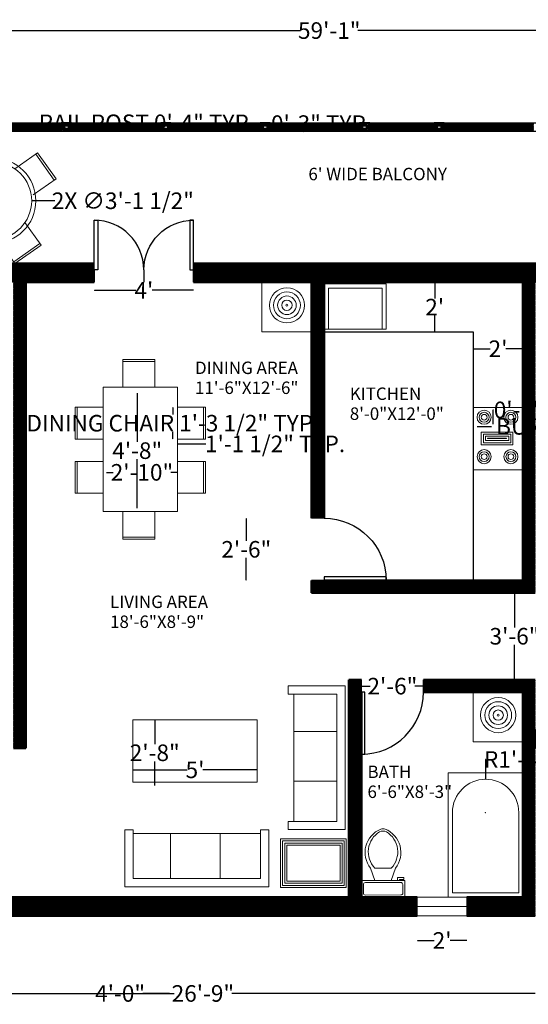
# Model space of a CAD drawing. Units: inches. Extents: x 348 to 1197, y 2602 to 3078.
# Tile 2 of 4: x 604 to 850, y 2602 to 3078. Entities that reach past the tile are written whole.
import ezdxf

# ---------------------------------------------------------------- set-up
doc = ezdxf.new("R2010")
doc.units = ezdxf.units.IN
doc.header["$MEASUREMENT"] = 0
for name, color, linetype, lineweight in [('A-ANNO-DIMS', 20, 'Continuous', 18), ('A-AREA-IDEN', 104, 'Continuous', 18), ('A-EQPM', 8, 'Continuous', 18), ('A-FLOR-CASE', 5, 'Continuous', 25), ('A-FLOR-FIXT', 9, 'Continuous', 18), ('A-WALL-PATT', 250, 'Continuous', 13), ('balcony', 201, 'Continuous', 25), ('doors', 1, 'Continuous', 25), ('sofa', 3, 'Continuous', 18), ('table', 6, 'Continuous', 18), ('walls', 4, 'Continuous', 50), ('windows', 2, 'Continuous', 18)]:
    doc.layers.add(name, color=color, linetype=linetype, lineweight=lineweight)
doc.styles.get("Standard").update_dxf_attribs({"font": 'arial.ttf'})
doc.dimstyles.get("Standard").update_dxf_attribs({"dimtxt": 8, "dimasz": 0.18, "dimexe": 0.18, "dimexo": 0.0625, "dimgap": 0.09, "dimtad": 0, "dimtih": 1, "dimtoh": 1, "dimdec": 0, "dimzin": 0, "dimdsep": 46, "dimlunit": 3, "dimtxsty": 'Standard', "dimblk": 'DOT', "dimcen": 0.09, "dimse1": 1, "dimse2": 1, "dimadec": 0, "dimazin": 0, "dimtfac": 1, "dimtdec": 0, "dimtofl": 0, "dimtmove": 0, "dimatfit": 3, "dimfxl": 1, "dimtolj": 1, "dimtzin": 0, "dimarcsym": 0})

# ---------------------------------------------------------------- blocks, each defined once
blk = doc.blocks.new('*U10')
for p, q in [((0, 0), (0, -6)), ((30, 0), (30, -6))]:
    blk.add_line(p, q)
blk.add_lwpolyline([(0, 0), (0, 30), (1.75, 30), (1.75, 0)], close=True)
blk.add_arc((0, 0), 30, 0, 90)
blk = doc.blocks.new('*U6')
for p, q in [((0, 0), (0, 6)), ((30, 0), (30, 6))]:
    blk.add_line(p, q)
blk.add_lwpolyline([(0, 0), (0, -30), (1.75, -30), (1.75, 0)], close=True)
blk.add_arc((0, 0), 30, 270, 0)
blk = doc.blocks.new('*U12')
for p, q in [((-4.02, 7.99), (-6.03, 13.99)), ((-4.03, 13.99), (3.97, 14.01)), ((3.98, 8.01), (5.97, 14.01)), ((6.98, 9.51), (9.98, 9.52)), ((6.98, 8.01), (6.98, 9.51)), ((9.98, 9.52), (9.98, 8.52)), ((-9.51, 5.98), (-9.5, 1.98)), ((9.98, 8.52), (7.98, 8.52)), ((7.98, 8.52), (7.98, 8.02))]:
    blk.add_line(p, q)
blk.add_lwpolyline([(-10.51, 7.98), (-10.5, -0.02), (10.5, 0.02), (10.48, 8.02)], close=True)
for points in [[(8.49, 7.02), (-8.51, 6.98)], [(9.5, 2.02), (9.49, 6.02)], [(-8.5, 0.98), (8.5, 1.02)]]:
    blk.add_lwpolyline(points)
for centre, radius, start, end in [((3.48, 21.59), 12.17, 112.136, 218.6382), ((4.16, 21.83), 11.33, 121.1605, 223.7396), ((-0.05, 27.88), 4, 65.8394, 114.3757), ((-0.05, 29), 4, 74.9681, 105.247), ((-3.56, 21.57), 12.17, 321.5766, 68.079), ((-4.24, 21.81), 11.33, 316.4753, 59.0544), ((-8.64, 6.11), 0.884, 81.9774, 188.2376), ((8.61, 6.14), 0.884, 351.9774, 98.2376), ((-8.63, 1.86), 0.884, 171.9774, 278.2376), ((8.62, 1.89), 0.884, 261.9774, 8.2376)]:
    blk.add_arc(centre, radius, start, end)
blk = doc.blocks.new('*U14')
at = {"layer": 'table'}
for p, q in [((-7.7, -6.73), (-7.7, 6.73)), ((-7.7, 6.73), (7.7, 6.73)), ((-7.7, 5.73), (7.7, 5.73)), ((7.7, 6.73), (7.7, -6.73))]:
    blk.add_line(p, q, dxfattribs=at)
blk = doc.blocks.new('*U15')
at = {"layer": 'table', "transparency": 16777216}
blk.add_blockref('*U14', (596.31, 3015.18), dxfattribs=at)
for p, rotation in [((570.95, 2992.17), 90), ((619.32, 2989.82), 270), ((593.96, 2966.81), 180)]:
    blk.add_blockref('*U14', p, dxfattribs=dict(at, rotation=rotation))
blk = doc.blocks.new('*U18')
for p, q in [((0, 0), (0, -6)), ((24, 0), (24, -6))]:
    blk.add_line(p, q)
blk.add_lwpolyline([(0, 0), (0, 24), (1.75, 24), (1.75, 0)], close=True)
blk.add_arc((0, 0), 24, 0, 90)
blk = doc.blocks.new('_Dot')
at = {"color": 0, "linetype": 'ByBlock', "lineweight": -2}
blk.add_line((-0.5, 0), (-1, 0), dxfattribs=at)
at = {"color": 0, "linetype": 'ByBlock', "const_width": 0.5}
blk.add_lwpolyline([(-0.25, 0, 1), (0.25, 0, 1)], format="xyb", close=True, dxfattribs=at)
blk = doc.blocks.new('*D25')
at = {"layer": 'A-ANNO-DIMS', "color": 0, "lineweight": -2, "transparency": 16777216}
for p, q in [((769.5, 2756.1), (773.53, 2756.1)), ((799.14, 2756.1), (795.11, 2756.1))]:
    blk.add_line(p, q, dxfattribs=at)
at = {"layer": 'Defpoints', "color": 0, "transparency": 16777216}
for p in [(769.32, 2756.1), (769.32, 2756.1), (799.32, 2756.2)]:
    blk.add_point(p, dxfattribs=at)
at = {"layer": 'A-ANNO-DIMS', "color": 0, "lineweight": -2, "transparency": 16777216, "xscale": 0.18, "yscale": 0.18, "zscale": 0.18, "rotation": 180}
blk.add_blockref('_Dot', (769.32, 2756.1), dxfattribs=at)
at = {"layer": 'A-ANNO-DIMS', "color": 0, "lineweight": -2, "transparency": 16777216, "xscale": 0.18, "yscale": 0.18, "zscale": 0.18}
blk.add_blockref('_Dot', (799.32, 2756.1), dxfattribs=at)
at = {"layer": 'A-ANNO-DIMS', "color": 0, "transparency": 16777216, "insert": (784.32, 2756.1), "char_height": 8, "attachment_point": 5}
blk.add_mtext('\\A1;2\'-6"', dxfattribs=at)
blk = doc.blocks.new('*D26')
at = {"layer": 'A-ANNO-DIMS', "color": 0, "lineweight": -2, "transparency": 16777216}
for p, q in [((843.28, 2801.02), (843.28, 2784.38)), ((843.28, 2759.38), (843.28, 2776.03))]:
    blk.add_line(p, q, dxfattribs=at)
at = {"layer": 'Defpoints', "color": 0, "transparency": 16777216}
for p in [(843.28, 2801.2), (843.28, 2759.2), (843.28, 2759.2)]:
    blk.add_point(p, dxfattribs=at)
at = {"layer": 'A-ANNO-DIMS', "color": 0, "lineweight": -2, "transparency": 16777216, "xscale": 0.18, "yscale": 0.18, "zscale": 0.18}
for p, rotation in [((843.28, 2801.2), 90), ((843.28, 2759.2), 270)]:
    blk.add_blockref('_Dot', p, dxfattribs=dict(at, rotation=rotation))
at = {"layer": 'A-ANNO-DIMS', "color": 0, "transparency": 16777216, "insert": (843.28, 2780.2), "char_height": 8, "attachment_point": 5}
blk.add_mtext('\\A1;3\'-6"', dxfattribs=at)
blk = doc.blocks.new('*D30')
at = {"layer": 'A-ANNO-DIMS', "color": 0, "lineweight": -2, "transparency": 16777216}
for p, q in [((640.5, 2947.32), (660.39, 2947.32)), ((688.14, 2947.32), (668.25, 2947.32))]:
    blk.add_line(p, q, dxfattribs=at)
at = {"layer": 'Defpoints', "color": 0, "transparency": 16777216}
for p in [(640.32, 2951.2), (688.32, 2951.2), (688.32, 2947.32)]:
    blk.add_point(p, dxfattribs=at)
at = {"layer": 'A-ANNO-DIMS', "color": 0, "lineweight": -2, "transparency": 16777216, "xscale": 0.18, "yscale": 0.18, "zscale": 0.18, "rotation": 180}
blk.add_blockref('_Dot', (640.32, 2947.32), dxfattribs=at)
at = {"layer": 'A-ANNO-DIMS', "color": 0, "lineweight": -2, "transparency": 16777216, "xscale": 0.18, "yscale": 0.18, "zscale": 0.18}
blk.add_blockref('_Dot', (688.32, 2947.32), dxfattribs=at)
at = {"layer": 'A-ANNO-DIMS', "color": 0, "transparency": 16777216, "insert": (664.32, 2947.32), "char_height": 8, "attachment_point": 5}
blk.add_mtext("\\A1;4'", dxfattribs=at)
blk = doc.blocks.new('*D31')
at = {"layer": 'A-ANNO-DIMS', "color": 0, "lineweight": -2, "transparency": 16777216}
for p, q in [((804.74, 2951.02), (804.74, 2943.31)), ((804.74, 2927.38), (804.74, 2935.1))]:
    blk.add_line(p, q, dxfattribs=at)
at = {"layer": 'Defpoints', "color": 0, "transparency": 16777216}
for p in [(798.02, 2951.2), (804.74, 2951.2), (798.02, 2927.2)]:
    blk.add_point(p, dxfattribs=at)
at = {"layer": 'A-ANNO-DIMS', "color": 0, "lineweight": -2, "transparency": 16777216, "xscale": 0.18, "yscale": 0.18, "zscale": 0.18}
for p, rotation in [((804.74, 2951.2), 90), ((804.74, 2927.2), 270)]:
    blk.add_blockref('_Dot', p, dxfattribs=dict(at, rotation=rotation))
at = {"layer": 'A-ANNO-DIMS', "color": 0, "transparency": 16777216, "insert": (804.74, 2939.2), "char_height": 8, "attachment_point": 5}
blk.add_mtext("\\A1;2'", dxfattribs=at)
blk = doc.blocks.new('*D32')
at = {"layer": 'A-ANNO-DIMS', "color": 0, "lineweight": -2, "transparency": 16777216}
for p, q in [((823.5, 2919.1), (831.48, 2919.1)), ((847.14, 2919.1), (839.16, 2919.1))]:
    blk.add_line(p, q, dxfattribs=at)
at = {"layer": 'Defpoints', "color": 0, "transparency": 16777216}
for p in [(823.32, 2927.2), (847.32, 2927.2), (847.32, 2919.1)]:
    blk.add_point(p, dxfattribs=at)
at = {"layer": 'A-ANNO-DIMS', "color": 0, "lineweight": -2, "transparency": 16777216, "xscale": 0.18, "yscale": 0.18, "zscale": 0.18, "rotation": 180}
blk.add_blockref('_Dot', (823.32, 2919.1), dxfattribs=at)
at = {"layer": 'A-ANNO-DIMS', "color": 0, "lineweight": -2, "transparency": 16777216, "xscale": 0.18, "yscale": 0.18, "zscale": 0.18}
blk.add_blockref('_Dot', (847.32, 2919.1), dxfattribs=at)
at = {"layer": 'A-ANNO-DIMS', "color": 0, "transparency": 16777216, "insert": (835.32, 2919.1), "char_height": 8, "attachment_point": 5}
blk.add_mtext("\\A1;2'", dxfattribs=at)
blk = doc.blocks.new('*D35')
at = {"layer": 'A-ANNO-DIMS', "color": 0, "lineweight": -2, "transparency": 16777216}
for p, q in [((659.18, 2715.69), (685.23, 2715.69)), ((718.82, 2715.69), (692.77, 2715.69))]:
    blk.add_line(p, q, dxfattribs=at)
at = {"layer": 'Defpoints', "color": 0, "transparency": 16777216}
for p in [(659, 2715.69), (659, 2709.77), (719, 2709.77)]:
    blk.add_point(p, dxfattribs=at)
at = {"layer": 'A-ANNO-DIMS', "color": 0, "lineweight": -2, "transparency": 16777216, "xscale": 0.18, "yscale": 0.18, "zscale": 0.18, "rotation": 180}
blk.add_blockref('_Dot', (659, 2715.69), dxfattribs=at)
at = {"layer": 'A-ANNO-DIMS', "color": 0, "lineweight": -2, "transparency": 16777216, "xscale": 0.18, "yscale": 0.18, "zscale": 0.18}
blk.add_blockref('_Dot', (719, 2715.69), dxfattribs=at)
at = {"layer": 'A-ANNO-DIMS', "color": 0, "transparency": 16777216, "insert": (689, 2715.69), "char_height": 8, "attachment_point": 5}
blk.add_mtext("\\A1;5'", dxfattribs=at)
blk = doc.blocks.new('*D36')
at = {"layer": 'A-ANNO-DIMS', "color": 0, "lineweight": -2, "transparency": 16777216}
for p, q in [((669.57, 2739.59), (669.57, 2728.1)), ((669.57, 2708.25), (669.57, 2719.75))]:
    blk.add_line(p, q, dxfattribs=at)
at = {"layer": 'Defpoints', "color": 0, "transparency": 16777216}
for p in [(669.57, 2739.77), (675.29, 2739.77), (673.39, 2708.07)]:
    blk.add_point(p, dxfattribs=at)
at = {"layer": 'A-ANNO-DIMS', "color": 0, "lineweight": -2, "transparency": 16777216, "xscale": 0.18, "yscale": 0.18, "zscale": 0.18}
for p, rotation in [((669.57, 2739.77), 90), ((669.57, 2708.07), 270)]:
    blk.add_blockref('_Dot', p, dxfattribs=dict(at, rotation=rotation))
at = {"layer": 'A-ANNO-DIMS', "color": 0, "transparency": 16777216, "insert": (669.57, 2723.92), "char_height": 8, "attachment_point": 5}
blk.add_mtext('\\A1;2\'-8"', dxfattribs=at)
blk = doc.blocks.new('*D37')
at = {"layer": 'A-ANNO-DIMS', "color": 0, "lineweight": -2, "transparency": 16777216}
for p, q in [((646.36, 2859.39), (649.5, 2859.39)), ((680.44, 2859.39), (677.3, 2859.39))]:
    blk.add_line(p, q, dxfattribs=at)
at = {"layer": 'Defpoints', "color": 0, "transparency": 16777216}
for p in [(646.18, 2869.07), (680.62, 2869.07), (646.18, 2859.39)]:
    blk.add_point(p, dxfattribs=at)
at = {"layer": 'A-ANNO-DIMS', "color": 0, "lineweight": -2, "transparency": 16777216, "xscale": 0.18, "yscale": 0.18, "zscale": 0.18, "rotation": 180}
blk.add_blockref('_Dot', (646.18, 2859.39), dxfattribs=at)
at = {"layer": 'A-ANNO-DIMS', "color": 0, "lineweight": -2, "transparency": 16777216, "xscale": 0.18, "yscale": 0.18, "zscale": 0.18}
blk.add_blockref('_Dot', (680.62, 2859.39), dxfattribs=at)
at = {"layer": 'A-ANNO-DIMS', "color": 0, "transparency": 16777216, "insert": (663.4, 2859.39), "char_height": 8, "attachment_point": 5}
blk.add_mtext('\\A1;2\'-10"', dxfattribs=at)
blk = doc.blocks.new('*D38')
at = {"layer": 'A-ANNO-DIMS', "color": 0, "lineweight": -2, "transparency": 16777216}
for p, q in [((661.12, 2897.52), (661.12, 2874.05)), ((661.12, 2842.23), (661.12, 2865.7))]:
    blk.add_line(p, q, dxfattribs=at)
at = {"layer": 'Defpoints', "color": 0, "transparency": 16777216}
for p in [(657.08, 2897.7), (661.12, 2897.7), (657.08, 2842.05)]:
    blk.add_point(p, dxfattribs=at)
at = {"layer": 'A-ANNO-DIMS', "color": 0, "lineweight": -2, "transparency": 16777216, "xscale": 0.18, "yscale": 0.18, "zscale": 0.18}
for p, rotation in [((661.12, 2897.7), 90), ((661.12, 2842.05), 270)]:
    blk.add_blockref('_Dot', p, dxfattribs=dict(at, rotation=rotation))
at = {"layer": 'A-ANNO-DIMS', "color": 0, "transparency": 16777216, "insert": (661.12, 2869.87), "char_height": 8, "attachment_point": 5}
blk.add_mtext('\\A1;4\'-8"', dxfattribs=at)
blk = doc.blocks.new('*D39')
at = {"layer": 'A-ANNO-DIMS', "color": 0, "lineweight": -2, "transparency": 16777216}
for p, q in [((796.5, 2633.23), (804.48, 2633.23)), ((820.14, 2633.23), (812.16, 2633.23))]:
    blk.add_line(p, q, dxfattribs=at)
at = {"layer": 'Defpoints', "color": 0, "transparency": 16777216}
for p in [(796.32, 2645.2), (820.32, 2645.2), (820.32, 2633.23)]:
    blk.add_point(p, dxfattribs=at)
at = {"layer": 'A-ANNO-DIMS', "color": 0, "lineweight": -2, "transparency": 16777216, "xscale": 0.18, "yscale": 0.18, "zscale": 0.18, "rotation": 180}
blk.add_blockref('_Dot', (796.32, 2633.23), dxfattribs=at)
at = {"layer": 'A-ANNO-DIMS', "color": 0, "lineweight": -2, "transparency": 16777216, "xscale": 0.18, "yscale": 0.18, "zscale": 0.18}
blk.add_blockref('_Dot', (820.32, 2633.23), dxfattribs=at)
at = {"layer": 'A-ANNO-DIMS', "color": 0, "transparency": 16777216, "insert": (808.32, 2633.23), "char_height": 8, "attachment_point": 5}
blk.add_mtext("\\A1;2'", dxfattribs=at)
blk = doc.blocks.new('RAIL-POST-CORE')
for points in [[(0, 0), (3, 0), (3, 3.9), (0, 3.9)], [(0.5, 0.5), (2.5, 0.5), (2.5, 3.4), (0.5, 3.4)], [(1, 1), (2, 1), (2, 2.9), (1, 2.9)]]:
    blk.add_lwpolyline(points, close=True)
blk = doc.blocks.new('DINING-CHAIR')
for p, q in [((0, 0), (0, 13.45)), ((0, 13.45), (15.39, 13.45)), ((0, 12.45), (15.39, 12.45)), ((15.39, 13.45), (15.39, 0))]:
    blk.add_line(p, q)
blk = doc.blocks.new('BALCONY-TABLE-ROUND')
for radius in [20.64, 18.64]:
    blk.add_circle((20.64, 20.64), radius)
blk = doc.blocks.new('BASIN-ROUND')
for radius in [8.49, 8.49, 8.49, 6.49, 4.49, 4.49, 2.49, 0.487]:
    blk.add_circle((8.49, 8.49), radius)
blk = doc.blocks.new('COOKTOP-BURNER')
for radius in [3.39, 2.39, 1.39]:
    blk.add_circle((3.39, 3.39), radius)
blk = doc.blocks.new('*D50')
at = {"layer": 'A-ANNO-DIMS', "color": 0, "lineweight": -2, "transparency": 16777216}
for p, q in [((720.96, 3028.25), (720.78, 3028.25)), ((724.68, 3028.25), (721.14, 3028.25))]:
    blk.add_line(p, q, dxfattribs=at)
at = {"layer": 'Defpoints', "color": 0, "transparency": 16777216}
for p in [(720.96, 3028.25), (720.96, 3027.67), (724.86, 3027.67)]:
    blk.add_point(p, dxfattribs=at)
at = {"layer": 'A-ANNO-DIMS', "color": 0, "lineweight": -2, "transparency": 16777216, "xscale": 0.18, "yscale": 0.18, "zscale": 0.18}
for p, rotation in [((720.96, 3028.25), 180.0000000000133), ((724.86, 3028.25), 1.33493e-11)]:
    blk.add_blockref('_Dot', p, dxfattribs=dict(at, rotation=rotation))
at = {"layer": 'A-ANNO-DIMS', "color": 0, "transparency": 16777216, "insert": (665.78, 3028.25), "char_height": 8, "attachment_point": 5}
blk.add_mtext('\\A1;RAIL POST 0\'-4" TYP.', dxfattribs=at)
blk = doc.blocks.new('*D51')
at = {"layer": 'A-ANNO-DIMS', "color": 0, "lineweight": -2, "transparency": 16777216}
for p, q in [((725.45, 3027.67), (725.45, 3027.85)), ((725.45, 3027.85), (725.63, 3027.85)), ((725.45, 3024.85), (725.45, 3027.49))]:
    blk.add_line(p, q, dxfattribs=at)
at = {"layer": 'Defpoints', "color": 0, "transparency": 16777216}
for p in [(724.86, 3027.67), (725.45, 3027.67), (724.86, 3024.67)]:
    blk.add_point(p, dxfattribs=at)
at = {"layer": 'A-ANNO-DIMS', "color": 0, "lineweight": -2, "transparency": 16777216, "xscale": 0.18, "yscale": 0.18, "zscale": 0.18}
for p, rotation in [((725.45, 3027.67), 90), ((725.45, 3024.67), 270)]:
    blk.add_blockref('_Dot', p, dxfattribs=dict(at, rotation=rotation))
at = {"layer": 'A-ANNO-DIMS', "color": 0, "transparency": 16777216, "insert": (750.1, 3027.85), "char_height": 8, "attachment_point": 5}
blk.add_mtext('\\A1;0\'-3" TYP.', dxfattribs=at)
blk = doc.blocks.new('*D56')
at = {"layer": 'A-ANNO-DIMS', "color": 0, "lineweight": -2, "transparency": 16777216}
for p, q in [((678.31, 2890.64), (678.31, 2887.35)), ((678.31, 2875.61), (678.31, 2878.89))]:
    blk.add_line(p, q, dxfattribs=at)
at = {"layer": 'Defpoints', "color": 0, "transparency": 16777216}
for p in [(680.62, 2890.82), (678.31, 2875.43), (680.62, 2875.43)]:
    blk.add_point(p, dxfattribs=at)
at = {"layer": 'A-ANNO-DIMS', "color": 0, "lineweight": -2, "transparency": 16777216, "xscale": 0.18, "yscale": 0.18, "zscale": 0.18}
for p, rotation in [((678.31, 2890.82), 90), ((678.31, 2875.43), 270)]:
    blk.add_blockref('_Dot', p, dxfattribs=dict(at, rotation=rotation))
at = {"layer": 'A-ANNO-DIMS', "color": 0, "transparency": 16777216, "insert": (678.31, 2883.12), "char_height": 8, "attachment_point": 5}
blk.add_mtext('\\A1;DINING CHAIR 1\'-3 1/2" TYP.', dxfattribs=at)
blk = doc.blocks.new('*D57')
at = {"layer": 'A-ANNO-DIMS', "color": 0, "lineweight": -2, "transparency": 16777216}
for p, q in [((680.8, 2873.12), (693.89, 2873.12)), ((694.07, 2873.12), (694.25, 2873.12))]:
    blk.add_line(p, q, dxfattribs=at)
at = {"layer": 'Defpoints', "color": 0, "transparency": 16777216}
for p in [(680.62, 2875.43), (694.07, 2875.43), (694.07, 2873.12)]:
    blk.add_point(p, dxfattribs=at)
at = {"layer": 'A-ANNO-DIMS', "color": 0, "lineweight": -2, "transparency": 16777216, "xscale": 0.18, "yscale": 0.18, "zscale": 0.18, "rotation": 180}
blk.add_blockref('_Dot', (680.62, 2873.12), dxfattribs=at)
at = {"layer": 'A-ANNO-DIMS', "color": 0, "lineweight": -2, "transparency": 16777216, "xscale": 0.18, "yscale": 0.18, "zscale": 0.18}
blk.add_blockref('_Dot', (694.07, 2873.12), dxfattribs=at)
at = {"layer": 'A-ANNO-DIMS', "color": 0, "transparency": 16777216, "insert": (727.67, 2873.12), "char_height": 8, "attachment_point": 5}
blk.add_mtext('\\A1;1\'-1 1/2" TYP.', dxfattribs=at)
blk = doc.blocks.new('*D62')
at = {"layer": 'A-ANNO-DIMS', "color": 0, "lineweight": -2, "transparency": 16777216}
for p, q in [((825.4, 2881.58), (831.83, 2881.58)), ((832.01, 2881.58), (832.19, 2881.58))]:
    blk.add_line(p, q, dxfattribs=at)
at = {"layer": 'Defpoints', "color": 0, "transparency": 16777216}
for p in [(825.22, 2882.6), (832.01, 2882.6), (832.01, 2881.58)]:
    blk.add_point(p, dxfattribs=at)
at = {"layer": 'A-ANNO-DIMS', "color": 0, "lineweight": -2, "transparency": 16777216, "xscale": 0.18, "yscale": 0.18, "zscale": 0.18, "rotation": 180}
blk.add_blockref('_Dot', (825.22, 2881.58), dxfattribs=at)
at = {"layer": 'A-ANNO-DIMS', "color": 0, "lineweight": -2, "transparency": 16777216, "xscale": 0.18, "yscale": 0.18, "zscale": 0.18}
blk.add_blockref('_Dot', (832.01, 2881.58), dxfattribs=at)
at = {"layer": 'A-ANNO-DIMS', "color": 0, "transparency": 16777216, "insert": (881.63, 2881.58), "char_height": 8, "attachment_point": 5}
blk.add_mtext('\\A1;BURNER 0\'-7" TYP.', dxfattribs=at)
blk = doc.blocks.new('*D63')
at = {"layer": 'A-ANNO-DIMS', "color": 0, "lineweight": -2, "transparency": 16777216}
for p, q in [((833.03, 2889.38), (833.03, 2889.56)), ((833.03, 2889.56), (833.21, 2889.56)), ((833.03, 2882.78), (833.03, 2889.2))]:
    blk.add_line(p, q, dxfattribs=at)
at = {"layer": 'Defpoints', "color": 0, "transparency": 16777216}
for p in [(832.01, 2889.38), (833.03, 2889.38), (832.01, 2882.6)]:
    blk.add_point(p, dxfattribs=at)
at = {"layer": 'A-ANNO-DIMS', "color": 0, "lineweight": -2, "transparency": 16777216, "xscale": 0.18, "yscale": 0.18, "zscale": 0.18}
for p, rotation in [((833.03, 2889.38), 90), ((833.03, 2882.6), 270)]:
    blk.add_blockref('_Dot', p, dxfattribs=dict(at, rotation=rotation))
at = {"layer": 'A-ANNO-DIMS', "color": 0, "transparency": 16777216, "insert": (857.68, 2889.56), "char_height": 8, "attachment_point": 5}
blk.add_mtext('\\A1;0\'-7" TYP.', dxfattribs=at)
blk = doc.blocks.new('*D68')
at = {"layer": 'A-ANNO-DIMS', "color": 0, "lineweight": -2, "transparency": 16777216}
for p, q in [((399.5, 3072.8), (739.99, 3072.8)), ((1108.14, 3072.8), (767.65, 3072.8))]:
    blk.add_line(p, q, dxfattribs=at)
at = {"layer": 'Defpoints', "color": 0, "transparency": 16777216}
for p in [(1108.32, 3072.8), (1108.32, 3028.2), (399.32, 3018.2)]:
    blk.add_point(p, dxfattribs=at)
at = {"layer": 'A-ANNO-DIMS', "color": 0, "lineweight": -2, "transparency": 16777216, "xscale": 0.18, "yscale": 0.18, "zscale": 0.18, "rotation": 180}
blk.add_blockref('_Dot', (399.32, 3072.8), dxfattribs=at)
at = {"layer": 'A-ANNO-DIMS', "color": 0, "lineweight": -2, "transparency": 16777216, "xscale": 0.18, "yscale": 0.18, "zscale": 0.18}
blk.add_blockref('_Dot', (1108.32, 3072.8), dxfattribs=at)
at = {"layer": 'A-ANNO-DIMS', "color": 0, "transparency": 16777216, "insert": (753.82, 3072.8), "char_height": 8, "attachment_point": 5}
blk.add_mtext('\\A1;59\'-1"', dxfattribs=at)
blk = doc.blocks.new('*D72')
at = {"layer": 'A-ANNO-DIMS', "color": 0, "lineweight": -2, "transparency": 16777216}
for p, q in [((532.5, 2607.65), (678.92, 2607.65)), ((853.14, 2607.65), (706.72, 2607.65))]:
    blk.add_line(p, q, dxfattribs=at)
at = {"layer": 'Defpoints', "color": 0, "transparency": 16777216}
for p in [(532.32, 2645.2), (853.32, 2645.2), (853.32, 2607.65)]:
    blk.add_point(p, dxfattribs=at)
at = {"layer": 'A-ANNO-DIMS', "color": 0, "lineweight": -2, "transparency": 16777216, "xscale": 0.18, "yscale": 0.18, "zscale": 0.18, "rotation": 180}
blk.add_blockref('_Dot', (532.32, 2607.65), dxfattribs=at)
at = {"layer": 'A-ANNO-DIMS', "color": 0, "lineweight": -2, "transparency": 16777216, "xscale": 0.18, "yscale": 0.18, "zscale": 0.18}
blk.add_blockref('_Dot', (853.32, 2607.65), dxfattribs=at)
at = {"layer": 'A-ANNO-DIMS', "color": 0, "transparency": 16777216, "insert": (692.82, 2607.65), "char_height": 8, "attachment_point": 5}
blk.add_mtext('\\A1;26\'-9"', dxfattribs=at)
blk = doc.blocks.new('*D76')
at = {"layer": 'A-ANNO-DIMS', "color": 0, "lineweight": -2, "transparency": 16777216}
for p, q in [((629.04, 2607.65), (641.98, 2607.65)), ((676.68, 2607.65), (663.75, 2607.65))]:
    blk.add_line(p, q, dxfattribs=at)
at = {"layer": 'Defpoints', "color": 0, "transparency": 16777216}
for p in [(628.86, 3024.67), (676.86, 3024.67), (676.86, 2607.65)]:
    blk.add_point(p, dxfattribs=at)
at = {"layer": 'A-ANNO-DIMS', "color": 0, "lineweight": -2, "transparency": 16777216, "xscale": 0.18, "yscale": 0.18, "zscale": 0.18, "rotation": 180}
blk.add_blockref('_Dot', (628.86, 2607.65), dxfattribs=at)
at = {"layer": 'A-ANNO-DIMS', "color": 0, "lineweight": -2, "transparency": 16777216, "xscale": 0.18, "yscale": 0.18, "zscale": 0.18}
blk.add_blockref('_Dot', (676.86, 2607.65), dxfattribs=at)
at = {"layer": 'A-ANNO-DIMS', "color": 0, "transparency": 16777216, "insert": (652.86, 2607.65), "char_height": 8, "attachment_point": 5}
blk.add_mtext('\\A1;4\'-0"', dxfattribs=at)
blk = doc.blocks.new('*D77')
at = {"layer": 'A-ANNO-DIMS', "color": 0, "lineweight": -2, "transparency": 16777216}
for p, q in [((713.77, 2837.02), (713.77, 2826.38)), ((713.77, 2807.38), (713.77, 2818.03))]:
    blk.add_line(p, q, dxfattribs=at)
at = {"layer": 'Defpoints', "color": 0, "transparency": 16777216}
for p in [(713.77, 2837.2), (751.32, 2837.2), (751.32, 2807.2)]:
    blk.add_point(p, dxfattribs=at)
at = {"layer": 'A-ANNO-DIMS', "color": 0, "lineweight": -2, "transparency": 16777216, "xscale": 0.18, "yscale": 0.18, "zscale": 0.18}
for p, rotation in [((713.77, 2837.2), 90), ((713.77, 2807.2), 270)]:
    blk.add_blockref('_Dot', p, dxfattribs=dict(at, rotation=rotation))
at = {"layer": 'A-ANNO-DIMS', "color": 0, "transparency": 16777216, "insert": (713.77, 2822.2), "char_height": 8, "attachment_point": 5}
blk.add_mtext('\\A1;2\'-6"', dxfattribs=at)
blk = doc.blocks.new('*D82')
at = {"layer": 'A-ANNO-DIMS', "color": 0, "lineweight": -2, "transparency": 16777216}
for p, q in [((591.41, 2990.59), (591.59, 2990.59)), ((591.5, 2990.5), (591.5, 2990.68)), ((621.33, 2990.59), (610.32, 2990.59))]:
    blk.add_line(p, q, dxfattribs=at)
at = {"layer": 'Defpoints', "color": 0, "transparency": 16777216}
for p in [(572.87, 2990.6), (610.14, 2990.59)]:
    blk.add_point(p, dxfattribs=at)
at = {"layer": 'A-ANNO-DIMS', "color": 0, "lineweight": -2, "transparency": 16777216, "xscale": 0.18, "yscale": 0.18, "zscale": 0.18, "rotation": 179.9894899347775}
blk.add_blockref('_Dot', (610.14, 2990.59), dxfattribs=at)
at = {"layer": 'A-ANNO-DIMS', "color": 0, "transparency": 16777216, "insert": (654.17, 2990.59), "char_height": 8, "attachment_point": 5}
blk.add_mtext('\\A1;2X ∅3\'-1 1/2"', dxfattribs=at)
blk = doc.blocks.new('*D83')
at = {"layer": 'A-ANNO-DIMS', "color": 0, "lineweight": -2, "transparency": 16777216}
for p, q in [((829.5, 2720.69), (829.32, 2720.69)), ((829.32, 2720.69), (829.32, 2711.27)), ((829.23, 2695.09), (829.41, 2695.09)), ((829.32, 2695), (829.32, 2695.18))]:
    blk.add_line(p, q, dxfattribs=at)
at = {"layer": 'Defpoints', "color": 0, "transparency": 16777216}
for p in [(829.32, 2711.09), (829.32, 2695.09)]:
    blk.add_point(p, dxfattribs=at)
at = {"layer": 'A-ANNO-DIMS', "color": 0, "lineweight": -2, "transparency": 16777216, "xscale": 0.18, "yscale": 0.18, "zscale": 0.18, "rotation": 269.9894074428831}
blk.add_blockref('_Dot', (829.32, 2711.09), dxfattribs=at)
at = {"layer": 'A-ANNO-DIMS', "color": 0, "transparency": 16777216, "insert": (844.05, 2720.69), "char_height": 8, "attachment_point": 5}
blk.add_mtext('\\A1;R1\'-4"', dxfattribs=at)

msp = doc.modelspace()

# ---------------------------------------------------------------- hatches: boundary and pattern name
at = {"layer": 'A-WALL-PATT'}
h = msp.add_hatch(dxfattribs=at)
h.set_pattern_fill('ANSI31', color=256, scale=1.5)
h.paths.add_polyline_path([(481.32, 2951.2), (509.32, 2951.2), (509.32, 2960.2), (505.32, 2960.2), (481.32, 2960.2), (481.32, 3018.2), (452.32, 3018.2), (452.32, 3009.2), (472.32, 3009.2), (472.32, 2943.2), (481.32, 2943.2)], flags=17)
h.paths.add_polyline_path([(428.32, 3018.2), (399.32, 3018.2), (399.32, 2904.2), (472.32, 2904.2), (472.32, 2726.2), (532.32, 2726.2), (532.32, 2696.2), (541.32, 2696.2), (541.32, 2726.2), (565.32, 2726.2), (565.32, 2735.2), (481.32, 2735.2), (481.32, 2758.72), (481.32, 2809.83), (481.31, 2809.83), (481.31, 2824.34), (481.31, 2884.34), (481.31, 2884.34), (481.31, 2898.86), (481.32, 2913.2), (472.32, 2913.2), (408.32, 2913.2), (408.32, 3009.2), (428.32, 3009.2)])
h.paths.add_polyline_path([(796.32, 2654.2), (769.32, 2654.2), (769.32, 2753.2), (769.32, 2759.2), (763.32, 2759.2), (763.32, 2735.2), (763.32, 2654.2), (541.32, 2654.2), (532.32, 2654.2), (532.32, 2645.2), (796.32, 2645.2)])
h.paths.add_polyline_path([(853.32, 2726.2), (1018.32, 2726.2), (1018.32, 2703.7), (1027.32, 2703.7), (1027.32, 2729.2), (1057.32, 2729.2), (1057.32, 2735.2), (919.32, 2735.2), (919.32, 2758.72), (919.32, 2765.2), (913.32, 2765.2), (913.32, 2735.2), (853.32, 2735.2), (853.32, 2759.2), (799.32, 2759.2), (799.32, 2753.2), (847.32, 2753.2), (847.32, 2654.2), (820.32, 2654.2), (820.32, 2645.2), (853.32, 2645.2)])
h.paths.add_polyline_path([(640.32, 2960.2), (577.32, 2960.2), (577.32, 2951.2), (601.32, 2951.2), (601.32, 2735.2), (601.32, 2726.2), (607.32, 2726.2), (607.32, 2951.2), (640.32, 2951.2)])
h.paths.add_polyline_path([(877.32, 2960.2), (688.32, 2960.2), (688.32, 2951.2), (745.32, 2951.2), (745.32, 2837.2), (751.32, 2837.2), (751.32, 2951.2), (847.32, 2951.2), (847.32, 2807.2), (751.32, 2807.2), (745.32, 2807.2), (745.32, 2801.2), (853.32, 2801.2), (853.32, 2807.2), (853.32, 2951.2), (877.32, 2951.2)])
h.paths.add_polyline_path([(1003.32, 2960.2), (949.32, 2960.2), (949.32, 2951.2), (973.32, 2951.2), (973.32, 2807.2), (906.15, 2807.2), (893.32, 2807.2), (893.32, 2801.2), (913.32, 2801.2), (919.32, 2801.2), (955.32, 2801.2), (979.32, 2801.2), (979.32, 2951.2), (1003.32, 2951.2)])
h.paths.add_polyline_path([(1108.32, 2960.2), (1104.32, 2960.2), (1075.32, 2960.2), (1075.32, 2951.2), (1099.32, 2951.2), (1099.32, 2735.2), (1087.32, 2735.2), (1087.32, 2729.2), (1099.32, 2729.2), (1099.32, 2654.2), (1027.32, 2654.2), (1027.32, 2679.7), (1018.32, 2679.7), (1018.32, 2645.2), (1108.32, 2645.2)])
h.paths.add_polyline_path([(509.32, 2992.2), (505.32, 2992.2), (505.32, 2965.1), (509.32, 2965.1)], flags=16)
h.paths.add_polyline_path([(509.32, 3023.27), (505.32, 3023.27), (505.32, 2997.1), (509.32, 2997.1)])
h.paths.add_polyline_path([(576.46, 3028.2), (509.32, 3028.2), (509.32, 3024.2), (576.46, 3024.2)])
h.paths.add_polyline_path([(624.46, 3028.2), (581.36, 3028.2), (581.36, 3024.2), (624.46, 3024.2)])
h.paths.add_polyline_path([(672.46, 3028.2), (629.36, 3028.2), (629.36, 3024.2), (672.46, 3024.2)])
h.paths.add_polyline_path([(720.46, 3028.2), (677.36, 3028.2), (677.36, 3024.2), (720.46, 3024.2)])
h.paths.add_polyline_path([(768.46, 3028.2), (725.36, 3028.2), (725.36, 3024.2), (768.46, 3024.2)])
h.paths.add_polyline_path([(804.46, 3028.2), (773.36, 3028.2), (773.36, 3024.2), (804.46, 3024.2)])
h.paths.add_polyline_path([(852.46, 3028.2), (809.36, 3028.2), (809.36, 3024.2), (852.46, 3024.2)])
h.paths.add_polyline_path([(900.46, 3028.2), (857.36, 3028.2), (857.36, 3024.2), (900.46, 3024.2)])
h.paths.add_polyline_path([(948.46, 3028.2), (905.36, 3028.2), (905.36, 3024.2), (948.46, 3024.2)])
h.paths.add_polyline_path([(996.46, 3028.2), (953.36, 3028.2), (953.36, 3024.2), (996.46, 3024.2)])
h.paths.add_polyline_path([(1056.46, 3028.2), (1001.36, 3028.2), (1001.36, 3024.2), (1056.46, 3024.2)])
h.paths.add_polyline_path([(1103.42, 3028.2), (1061.36, 3028.2), (1061.36, 3024.2), (1103.42, 3024.2)])
h.paths.add_polyline_path([(1108.32, 3024.17), (1104.32, 3024.17), (1104.32, 2994.89), (1108.32, 2994.89)])
h.paths.add_polyline_path([(1108.32, 2989.99), (1104.32, 2989.99), (1104.32, 2965.1), (1108.32, 2965.1)])

# ---------------------------------------------------------------- linework, layer by layer
at = {"layer": 'A-EQPM'}
for p, q in [((823.32, 2890.63), (847.32, 2890.63)), ((823.32, 2860.63), (847.32, 2860.63))]:
    msp.add_line(p, q, dxfattribs=at)
for points in [[(827.23, 2878.82), (842.49, 2878.82), (842.49, 2872.7), (827.23, 2872.7)], [(828.23, 2877.82), (841.49, 2877.82), (841.49, 2873.7), (828.23, 2873.7)], [(829.23, 2876.82), (840.49, 2876.82), (840.49, 2874.7), (829.23, 2874.7)], [(830.23, 2875.82), (839.49, 2875.82), (839.49, 2875.7), (830.23, 2875.7)]]:
    msp.add_lwpolyline(points, close=True, dxfattribs=at)
msp.add_circle((828.62, 2866.96), 3.39, dxfattribs=at)
at = {"layer": 'A-FLOR-CASE'}
for p, q in [((751.32, 2927.2), (823.32, 2927.2)), ((823.32, 2927.2), (823.32, 2807.2))]:
    msp.add_line(p, q, dxfattribs=at)
at = {"layer": 'A-FLOR-FIXT'}
for p, q in [((721.32, 2927.2), (721.32, 2951.2)), ((781.32, 2950.39), (751.52, 2950.39)), ((751.52, 2950.39), (751.52, 2928.58)), ((781.32, 2928.58), (781.32, 2950.39)), ((779.32, 2948.39), (753.52, 2948.39)), ((753.52, 2948.39), (753.52, 2928.58)), ((779.32, 2928.58), (779.32, 2948.39)), ((745.32, 2927.2), (721.32, 2927.2)), ((751.52, 2928.58), (781.32, 2928.58)), ((823.32, 2729.2), (823.32, 2753.2)), ((847.32, 2729.2), (823.32, 2729.2)), ((847.32, 2714.2), (811.32, 2714.2)), ((811.32, 2714.2), (811.32, 2654.2)), ((847.32, 2654.2), (847.32, 2714.2)), ((813.32, 2695.09), (813.32, 2656.2)), ((845.32, 2656.2), (845.32, 2695.09)), ((813.32, 2656.2), (845.32, 2656.2))]:
    msp.add_line(p, q, dxfattribs=at)
msp.add_arc((829.32, 2695.09), 16, 0, 180, dxfattribs=at)
at = {"layer": 'balcony'}
for p, q in [((505.32, 3028.2), (1108.32, 3028.2)), ((509.32, 3024.2), (1104.32, 3024.2))]:
    msp.add_line(p, q, dxfattribs=at)
for points in [[(629.36, 3024.17), (629.36, 3028.17), (624.46, 3028.17), (624.46, 3024.17)], [(677.36, 3024.17), (677.36, 3028.17), (672.46, 3028.17), (672.46, 3024.17)], [(725.36, 3024.17), (725.36, 3028.17), (720.46, 3028.17), (720.46, 3024.17)], [(773.36, 3024.17), (773.36, 3028.17), (768.46, 3028.17), (768.46, 3024.17)], [(809.36, 3024.17), (809.36, 3028.17), (804.46, 3028.17), (804.46, 3024.17)]]:
    msp.add_lwpolyline(points, close=True, dxfattribs=at)
at = {"layer": 'doors'}
for p, q in [((640.32, 2951.2), (640.32, 2960.2)), ((688.32, 2951.2), (688.32, 2960.2)), ((751.32, 2837.2), (745.32, 2837.2)), ((751.32, 2807.2), (745.32, 2807.2)), ((769.32, 2753.2), (769.32, 2759.2)), ((799.32, 2753.2), (799.32, 2759.2))]:
    msp.add_line(p, q, dxfattribs=at)
at = {"layer": 'sofa'}
for p, q in [((733.91, 2752.26), (733.91, 2756.26)), ((733.91, 2752.26), (757.44, 2752.26)), ((736.77, 2752.26), (736.77, 2690.77)), ((736.77, 2734.26), (757.44, 2734.26)), ((736.77, 2710.26), (757.44, 2710.26)), ((659.15, 2686.64), (659.15, 2663.11)), ((659.15, 2684.89), (720.63, 2684.89)), ((677.15, 2684.89), (677.15, 2663.11)), ((701.15, 2684.89), (701.15, 2663.11)), ((724.63, 2686.64), (720.63, 2686.64))]:
    msp.add_line(p, q, dxfattribs=at)
for points in [[(733.91, 2756.26), (761.44, 2756.26), (761.44, 2686.77), (733.91, 2686.77), (733.91, 2690.77), (757.44, 2690.77), (757.44, 2752.26), (733.91, 2752.26)], [(724.63, 2686.64), (724.63, 2659.11), (655.15, 2659.11), (655.15, 2686.64), (659.15, 2686.64), (659.15, 2663.11), (720.63, 2663.11), (720.63, 2686.64)]]:
    msp.add_lwpolyline(points, dxfattribs=at)
at = {"layer": 'table'}
for p, q in [((644.62, 2900.5), (680.62, 2900.5)), ((644.62, 2840.5), (644.62, 2900.5)), ((680.62, 2900.5), (680.62, 2840.5)), ((680.62, 2840.5), (644.62, 2840.5)), ((659, 2739.77), (719, 2739.77)), ((659, 2709.77), (659, 2739.77)), ((719, 2739.77), (719, 2709.77)), ((719, 2709.77), (659, 2709.77))]:
    msp.add_line(p, q, dxfattribs=at)
for points in [[(762.02, 2658.87), (730.31, 2658.87), (730.31, 2682.32), (762.02, 2682.32)], [(761.02, 2659.87), (731.31, 2659.87), (731.31, 2681.32), (761.02, 2681.32)], [(760.02, 2660.87), (732.31, 2660.87), (732.31, 2680.32), (760.02, 2680.32)], [(759.02, 2661.87), (733.31, 2661.87), (733.31, 2679.32), (759.02, 2679.32)]]:
    msp.add_lwpolyline(points, close=True, dxfattribs=at)
at = {"layer": 'walls'}
for p, q in [((577.32, 2960.2), (640.32, 2960.2)), ((688.32, 2960.2), (877.32, 2960.2)), ((607.32, 2951.2), (607.32, 2726.2)), ((607.32, 2951.2), (640.32, 2951.2)), ((688.32, 2951.2), (745.32, 2951.2)), ((745.32, 2951.2), (745.32, 2837.2)), ((751.32, 2951.2), (751.32, 2837.2)), ((751.32, 2951.2), (847.32, 2951.2)), ((847.32, 2951.2), (847.32, 2807.2)), ((745.32, 2807.2), (745.32, 2801.2)), ((751.32, 2807.2), (847.32, 2807.2)), ((745.32, 2801.2), (853.32, 2801.2)), ((763.32, 2735.2), (763.32, 2759.2)), ((763.32, 2759.2), (769.32, 2759.2)), ((799.32, 2759.2), (853.32, 2759.2)), ((769.32, 2753.2), (769.32, 2654.2)), ((799.32, 2753.2), (847.32, 2753.2)), ((847.32, 2753.2), (847.32, 2654.2)), ((763.32, 2735.2), (763.32, 2654.2)), ((601.32, 2726.2), (607.32, 2726.2)), ((541.32, 2654.2), (763.32, 2654.2)), ((769.32, 2654.2), (796.32, 2654.2)), ((820.32, 2654.2), (847.32, 2654.2)), ((532.32, 2645.2), (796.32, 2645.2)), ((820.32, 2645.2), (853.32, 2645.2))]:
    msp.add_line(p, q, dxfattribs=at)
at = {"layer": 'windows'}
for p, q in [((796.32, 2654.2), (796.32, 2645.2)), ((796.32, 2654.2), (820.32, 2654.2)), ((820.32, 2654.2), (820.32, 2645.2)), ((820.32, 2649.7), (796.32, 2649.7)), ((796.32, 2645.2), (820.32, 2645.2))]:
    msp.add_line(p, q, dxfattribs=at)

# ---------------------------------------------------------------- block references
at = {"layer": 'A-EQPM'}
for p in [(825.22, 2882.6), (838.14, 2882.6)]:
    msp.add_blockref('COOKTOP-BURNER', p, dxfattribs=at)
at = {"layer": 'A-EQPM', "rotation": 75.96375653207353}
for p in [(831.09, 2862.85), (844, 2862.85)]:
    msp.add_blockref('COOKTOP-BURNER', p, dxfattribs=at)
at = {"layer": 'A-FLOR-FIXT'}
for name, p in [('BASIN-ROUND', (724.91, 2931.61)), ('BASIN-ROUND', (826.91, 2733.61)), ('*U12', (779.82, 2654.2))]:
    msp.add_blockref(name, p, dxfattribs=at)
at = {"layer": 'balcony', "rotation": 90.00000000001351}
for p in [(628.86, 3024.67), (676.86, 3024.67), (724.86, 3024.67), (772.86, 3024.67), (808.86, 3024.67)]:
    msp.add_blockref('RAIL-POST-CORE', p, dxfattribs=at)
at = {"layer": 'doors'}
for name, p in [('*U18', (640.32, 2957.2)), ('*U6', (769.32, 2753.2))]:
    msp.add_blockref(name, p, dxfattribs=at)
at = {"layer": 'doors', "xscale": -1}
msp.add_blockref('*U18', (688.32, 2957.2), dxfattribs=at)
at = {"layer": 'doors', "xscale": -1, "rotation": 270}
msp.add_blockref('*U10', (751.32, 2807.2), dxfattribs=at)
at = {"layer": 'table'}
for name, p, rotation in [('*U15', (-644.77, 5778.4), 215.168770522954), ('DINING-CHAIR', (644.62, 2875.43), 89.9999999999992), ('DINING-CHAIR', (680.62, 2890.82), 270.0000000000011), ('DINING-CHAIR', (644.62, 2849.27), 90.00000000000081), ('DINING-CHAIR', (680.62, 2864.66), 270.0000000000045), ('DINING-CHAIR', (669.61, 2840.5), 180)]:
    msp.add_blockref(name, p, dxfattribs=dict(at, rotation=rotation))
for name, p in [('BALCONY-TABLE-ROUND', (570.87, 2969.95)), ('DINING-CHAIR', (654.21, 2900.5))]:
    msp.add_blockref(name, p, dxfattribs=at)

# ---------------------------------------------------------------- texts
at = {"layer": 'A-AREA-IDEN'}
for s, p in [("6' WIDE BALCONY ", (743.75, 3000.49)), ('DINING AREA ', (689, 2906.88)), ('11\'-6"X12\'-6"', (689, 2897.24)), ('KITCHEN ', (763.75, 2894.37)), ('8\'-0"X12\'-0"', (763.75, 2884.73)), ('LIVING AREA ', (647.99, 2793.85)), ('18\'-6"X8\'-9"', (647.99, 2784.21)), ('BATH ', (772.28, 2711.72)), ('6\'-6"X8\'-3"', (772.28, 2702.08))]:
    msp.add_text(s, height=6, dxfattribs=at).set_placement(p)

# ---------------------------------------------------------------- dimensions: what is measured, and where the dimension line sits
at = {"layer": 'A-ANNO-DIMS'}
for base, p1, p2, override, picture, middle in [((1108.32, 3072.8), (399.32, 3018.2), (1108.32, 3028.2), {"dimdec": 1, "dimlfac": 1, "dimrnd": 0, "dimzin": 1, "dimdsep": 46, "dimlunit": 4, "dimfrac": 2}, '*D68', (753.82, 3072.8)), ((676.86, 2607.65), (628.86, 3024.67), (676.86, 3024.67), {"dimdec": 1, "dimlfac": 1, "dimrnd": 0, "dimzin": 1, "dimdsep": 46, "dimlunit": 4, "dimfrac": 2}, '*D76', (652.86, 2607.65)), ((688.32, 2947.32), (640.32, 2951.2), (688.32, 2951.2), {"dimclrd": 0, "dimclre": 0, "dimclrt": 0}, '*D30', (664.32, 2947.32)), ((847.32, 2919.1), (823.32, 2927.2), (847.32, 2927.2), {"dimclrd": 0, "dimclre": 0, "dimclrt": 0}, '*D32', (835.32, 2919.1)), ((646.18, 2859.39), (680.62, 2869.07), (646.18, 2869.07), {"dimclrd": 0, "dimclre": 0, "dimclrt": 0}, '*D37', (663.4, 2859.39)), ((769.32, 2756.1), (799.32, 2756.2), (769.32, 2756.1), {"dimclrd": 0, "dimclre": 0, "dimclrt": 0}, '*D25', (784.32, 2756.1)), ((659, 2715.69), (719, 2709.77), (659, 2709.77), {"dimclrd": 0, "dimclre": 0, "dimclrt": 0}, '*D35', (689, 2715.69)), ((853.32, 2607.65), (532.32, 2645.2), (853.32, 2645.2), {"dimdec": 1, "dimlfac": 1, "dimrnd": 0, "dimzin": 1, "dimdsep": 46, "dimlunit": 4, "dimfrac": 2}, '*D72', (692.82, 2607.65)), ((820.32, 2633.23), (796.32, 2645.2), (820.32, 2645.2), {"dimclrd": 0, "dimclre": 0, "dimclrt": 0}, '*D39', (808.32, 2633.23))]:
    dim = msp.add_linear_dim(base=base, p1=p1, p2=p2, dimstyle='Standard', override=override, dxfattribs=at)
    dim.commit()
    dim.dimension.update_dxf_attribs({"geometry": picture, "text_midpoint": middle})
for base, p1, p2, angle, text, picture, middle in [((720.96, 3028.25), (724.86, 3027.67), (720.96, 3027.67), 180, 'RAIL POST <> TYP.', '*D50', (665.78, 3028.25)), ((725.45, 3027.67), (724.86, 3024.67), (724.86, 3027.67), 90, '<> TYP.', '*D51', (750.1, 3027.85)), ((678.31, 2875.43), (680.62, 2890.82), (680.62, 2875.43), 270, 'DINING CHAIR <> TYP.', '*D56', (678.31, 2883.12)), ((833.03, 2889.38), (832.01, 2882.6), (832.01, 2889.38), 90, '<> TYP.', '*D63', (857.68, 2889.56)), ((694.0696, 2873.1182), (680.6191, 2875.4268), (694.0696, 2875.4268), 0, '<> TYP.', '*D57', (727.6657, 2873.1182))]:
    dim = msp.add_linear_dim(base=base, p1=p1, p2=p2, angle=angle, text=text, dimstyle='Standard', override={"dimdec": 1, "dimlfac": 1, "dimrnd": 0, "dimzin": 1, "dimdsep": 46, "dimlunit": 4, "dimfrac": 2}, dxfattribs=at)
    dim.commit()
    dim.dimension.update_dxf_attribs({"geometry": picture, "text_midpoint": middle})
dim = msp.add_diameter_dim_2p(p1=(572.87, 2990.6), p2=(610.14, 2990.59), text='2X <>', dimstyle='Standard', override={"dimdec": 1, "dimlfac": 1, "dimrnd": 0, "dimzin": 1, "dimdsep": 46, "dimlunit": 4, "dimfrac": 2}, dxfattribs=at)
dim.commit()
dim.dimension.update_dxf_attribs({"geometry": '*D82', "text_midpoint": (621.33, 2990.59), "dimtype": 163})
for base, p1, p2, override, picture, middle in [((804.74, 2951.2), (798.02, 2927.2), (798.02, 2951.2), {"dimclrd": 0, "dimclre": 0, "dimclrt": 0}, '*D31', (804.74, 2939.2)), ((661.12, 2897.7), (657.08, 2842.05), (657.08, 2897.7), {"dimclrd": 0, "dimclre": 0, "dimclrt": 0}, '*D38', (661.12, 2869.87)), ((713.77, 2837.2), (751.32, 2807.2), (751.32, 2837.2), {"dimdec": 1, "dimlfac": 1, "dimrnd": 0, "dimzin": 1, "dimdsep": 46, "dimlunit": 4, "dimfrac": 2}, '*D77', (713.77, 2822.2)), ((843.28, 2759.2), (843.28, 2801.2), (843.28, 2759.2), {"dimclrd": 0, "dimclre": 0, "dimclrt": 0}, '*D26', (843.28, 2780.2)), ((669.57, 2739.77), (673.39, 2708.07), (675.29, 2739.77), {"dimclrd": 0, "dimclre": 0, "dimclrt": 0}, '*D36', (669.57, 2723.92))]:
    dim = msp.add_linear_dim(base=base, p1=p1, p2=p2, angle=90, dimstyle='Standard', override=override, dxfattribs=at)
    dim.commit()
    dim.dimension.update_dxf_attribs({"geometry": picture, "text_midpoint": middle})
dim = msp.add_linear_dim(base=(832.01, 2881.58), p1=(825.22, 2882.6), p2=(832.01, 2882.6), text='BURNER <> TYP.', dimstyle='Standard', override={"dimdec": 1, "dimlfac": 1, "dimrnd": 0, "dimzin": 1, "dimdsep": 46, "dimlunit": 4, "dimfrac": 2}, dxfattribs=at)
dim.commit()
dim.dimension.update_dxf_attribs({"geometry": '*D62', "text_midpoint": (881.63, 2881.58)})
dim = msp.add_radius_dim(center=(829.32, 2695.09), mpoint=(829.32, 2711.09), dimstyle='Standard', override={"dimdec": 1, "dimlfac": 1, "dimrnd": 0, "dimzin": 1, "dimdsep": 46, "dimlunit": 4, "dimfrac": 2}, dxfattribs=at)
dim.commit()
dim.dimension.update_dxf_attribs({"geometry": '*D83', "text_midpoint": (844.05, 2720.69), "dimtype": 164})

doc.saveas('drawing.dxf')
